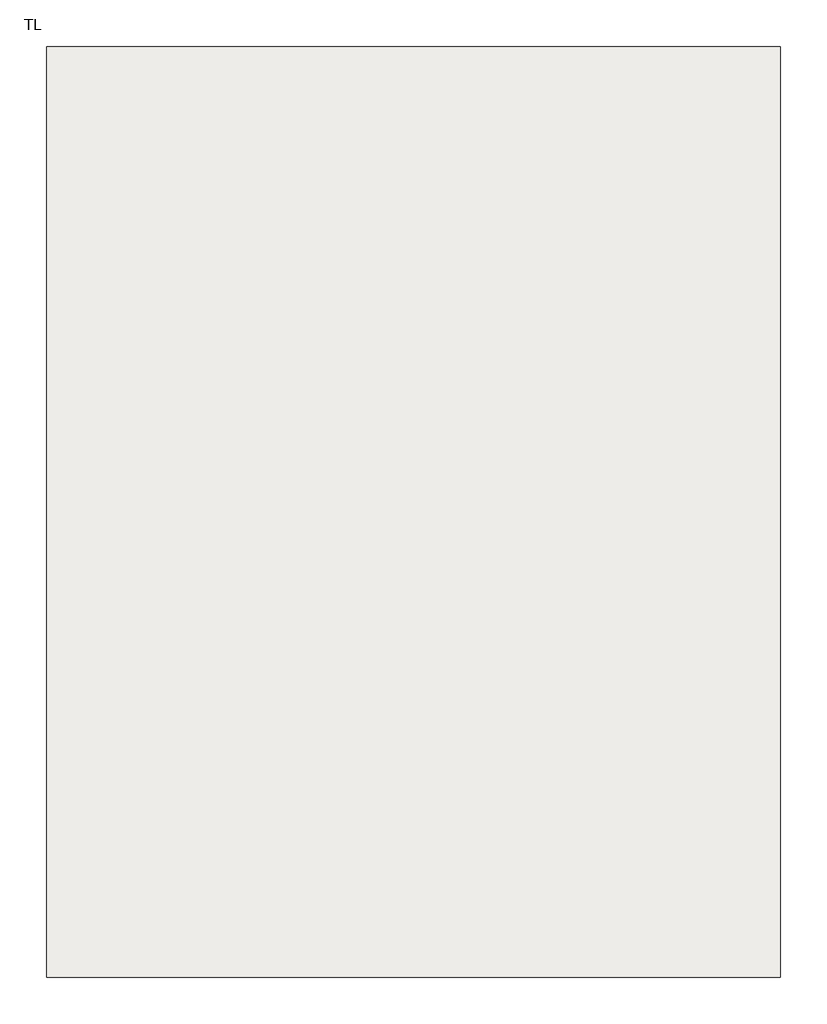
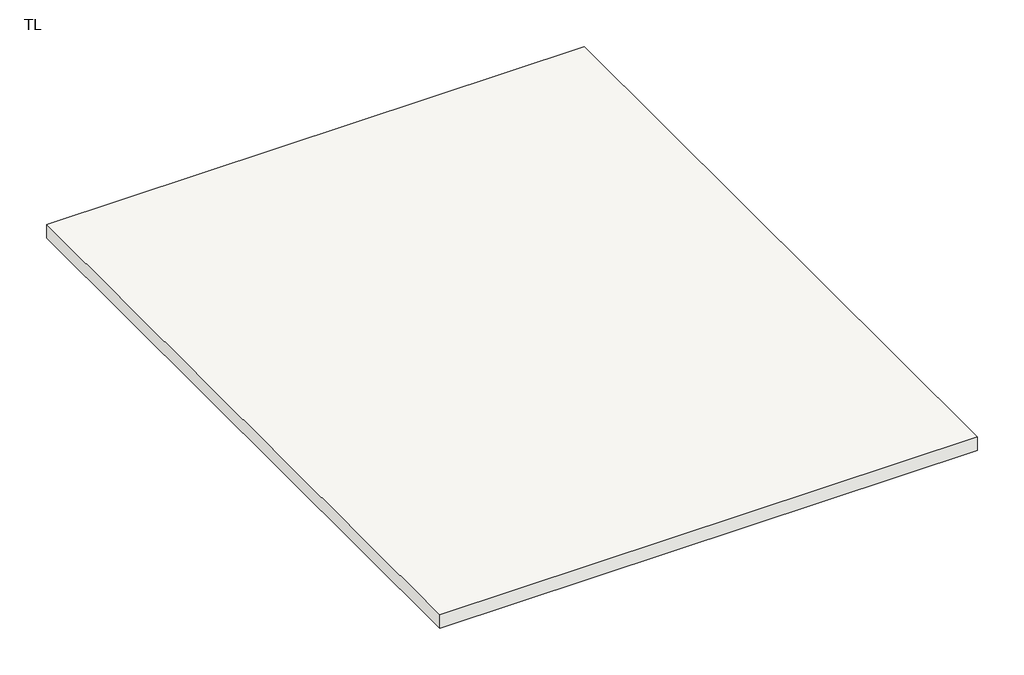
# One storey: 1 slab.
"""IFC4 building model written with IfcOpenShell, lengths in millimetres."""

from ifc_helpers import new_model, si_unit, frame, origin, place, context, project, spatial, polyline, outline, extrude, element, save

model = new_model("IFC4")

# Units and contexts
model_context = context("Model", 3, world=origin())
ifc_project = project(units=[si_unit("LENGTHUNIT", "METRE", prefix="MILLI")], contexts=[model_context])

# Site, building, storey
site = spatial("IfcSite", under=ifc_project)
building = spatial("IfcBuilding", under=site)
storey = spatial("IfcBuildingStorey", under=building, Name="TL", Elevation=9631.68)

# Slab
placement = place(None, origin())
element("IfcSlab", 1, ObjectType="RCC SLAB", at=placement, inside=storey, context=model_context, shape_type="SweptSolid", body=[
    extrude(outline(polyline([(-6495.4132565, -656.9593981), (-6495.4132565, -10219.6521308), (-14039.0335145, -10219.6521308), (-14039.0335145, -656.9593981), (-6495.4132565, -656.9593981)])), frame((0.0, 0.0, 9431.7312), z_axis=(0.0, 0.0, 1.0), x_axis=(1.0, 0.0, 0.0)), (0.0, 0.0, 1.0), 199.9488),
])

save(model, "model.ifc")

# Revit data of these elements
# Type "RCC SLAB"
#   Layers, outside or top first: 0.656 ft no material (function 1)
# Element 1 (IfcSlab, "RCC SLAB")
#   Height Offset From Level = 0.0 ft
#   built-in parameter 1001954 = 1
#   Phase Created = New Construction
